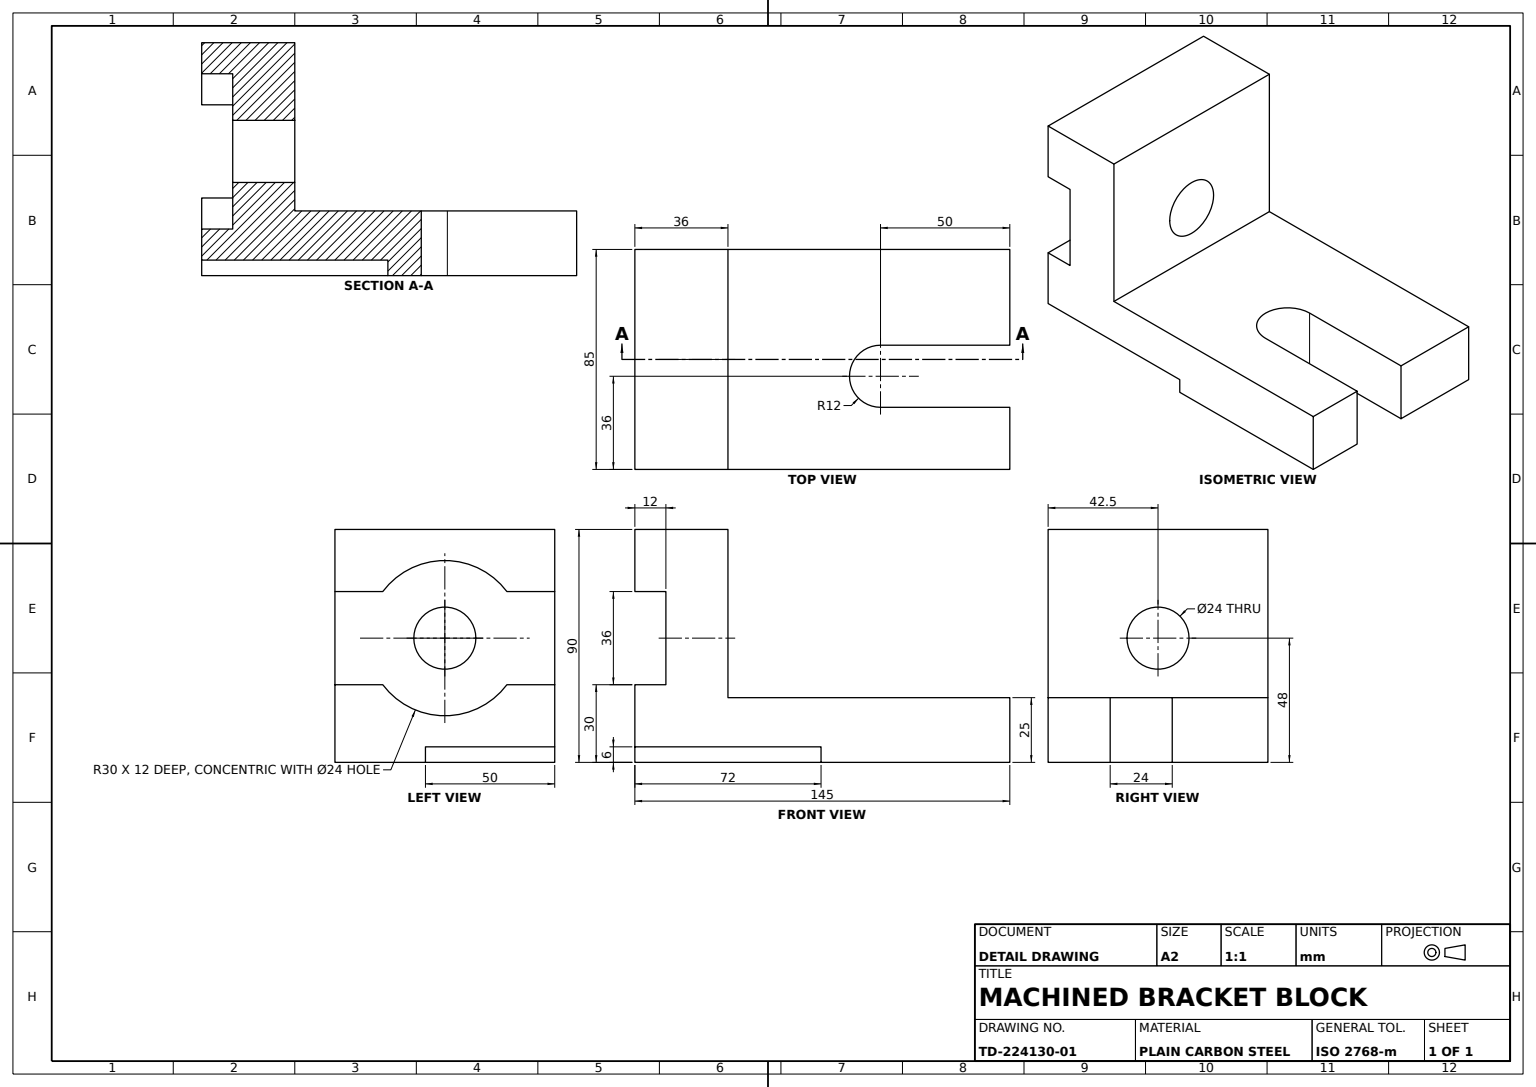
from build123d import *

# Parameters (mm, degrees)
FORKED_BLOCK_BODY_DEPTH      = 42.5
SLOT_12X24_DEPTH             = 85
RELIEF_GROOVE_SKETCH_W       = 72
RELIEF_GROOVE_SKETCH_H       = 6
BOTTOM_RELIEF_GROOVE_6_DEPTH = 50
BORE_AND_SADDLE_SKETCH_R     = 12
SADDLE_RECESS_48_DEPTH       = 12
BORE_24_REACH                = 177.873
SKETCH6_3_R                  = 12


with BuildPart() as part:
    # Block Profile Sketch → Forked Block Body (new, symmetric)
    with BuildSketch(Plane(origin=(0, 0, 0), x_dir=(0, 0, -1), z_dir=(1, 0, 0))):
        Polygon((50, 0), (-95, 0), (-95, 90), (-59, 90), (-59, 25), (50, 25), align=None)
    extrude(amount=FORKED_BLOCK_BODY_DEPTH, both=True)

    # Slot Sketch → Slot 12x24 (cut)
    with BuildSketch(Plane(origin=(0, 25, 0), x_dir=(1, 0, 0), z_dir=(0, 1, 0))):
        with BuildLine():
            Line((18.5, 0), (18.5, 50))
            Line((18.5, 50), (-5.5, 50))
            Line((-5.5, 50), (-5.5, 0))
            ThreePointArc((-5.5, 0), (6.5, -12), (18.5, 0))
        make_face()
    extrude(amount=-SLOT_12X24_DEPTH, mode=Mode.SUBTRACT)

    # Relief Groove Sketch → Bottom Relief Groove 6 (cut)
    with BuildSketch(Plane(origin=(42.5, 0, 0), x_dir=(0, 0, -1), z_dir=(1, 0, 0))):
        with Locations((-59, 3)):
            Rectangle(RELIEF_GROOVE_SKETCH_W, RELIEF_GROOVE_SKETCH_H)
    extrude(amount=-BOTTOM_RELIEF_GROOVE_6_DEPTH, mode=Mode.SUBTRACT)

    # Bore and Saddle Sketch → Saddle Recess _48 (cut)
    with BuildSketch(Plane.XY.offset(95)):
        with BuildLine():
            Line((-42.5, 66), (-42.5, 30))
            Line((-42.5, 30), (-24, 30))
            ThreePointArc((-24, 30), (0, 18), (24, 30))
            Line((24, 30), (42.5, 30))
            Line((42.5, 30), (42.5, 66))
            Line((42.5, 66), (24, 66))
            ThreePointArc((24, 66), (0, 78), (-24, 66))
            Line((-24, 66), (-42.5, 66))
        make_face()
        with Locations((0, 48)):
            Circle(BORE_AND_SADDLE_SKETCH_R, mode=Mode.SUBTRACT)
    extrude(amount=-SADDLE_RECESS_48_DEPTH, mode=Mode.SUBTRACT)

    # Sketch6_3 → Bore _24 (cut, up to next)
    with BuildSketch(Plane.XY.offset(95), mode=Mode.PRIVATE) as bore_24_sk1:
        with Locations((0, 48)):
            Circle(SKETCH6_3_R)
    bore_24_tool1 = extrude(bore_24_sk1.sketch, amount=-BORE_24_REACH, mode=Mode.PRIVATE) & part.part
    add(bore_24_tool1.solids().sort_by_distance((0, 48, 95))[0], mode=Mode.SUBTRACT)


solid = part.part
